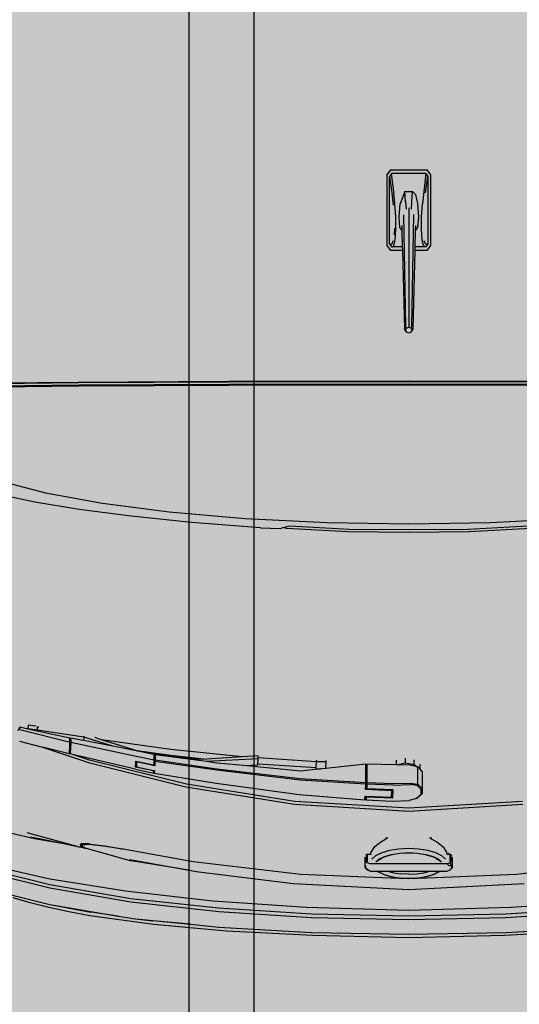
# Model space of a CAD drawing. Units: inches. Extents: x 1884 to 2398, y 474 to 1488.
# Tile 20 of 39: x 2308 to 2330, y 577 to 620. Entities that reach past the tile are written whole.
import ezdxf

# ---------------------------------------------------------------- set-up
doc = ezdxf.new("R2010")
doc.units = ezdxf.units.IN
doc.header["$MEASUREMENT"] = 0
doc.layers.get('0').update_dxf_attribs({"color": 250})
doc.layers.add('A-ANNO-DIMS', color=2, linetype='Continuous', lineweight=18)
doc.layers.add('C-VEHI', color=8, linetype='Continuous', lineweight=18)
doc.layers.add('Edges', color=250, linetype='Continuous')
doc.layers.add('L-PVMT-PATT', color=9, linetype='Continuous', lineweight=13, true_color=0xc7c8ca)
doc.styles.get("Standard").update_dxf_attribs({"font": 'arial.ttf'})
doc.dimstyles.get("Standard").update_dxf_attribs({"dimtxt": 7, "dimasz": 0.18, "dimexe": 0.18, "dimexo": 0.0625, "dimgap": 0.09, "dimtad": 0, "dimtih": 1, "dimtoh": 1, "dimzin": 0, "dimdsep": 46, "dimlunit": 3, "dimtxsty": 'Standard', "dimcen": 0.09, "dimadec": 0, "dimazin": 0, "dimtfac": 1, "dimtofl": 0, "dimtmove": 0, "dimatfit": 3, "dimfxl": 1, "dimtolj": 1, "dimtzin": 0, "dimarcsym": 0})

# ---------------------------------------------------------------- blocks, each defined once
blk = doc.blocks.new('Nissan Qashqai pl')
at = {"layer": 'Edges'}
for p, q in [((11.5963, 12.0406), (11.5823, 12.1589)), ((11.626, 12.1375), (11.6329, 12.0344)), ((11.6399, 12.029), (11.6333, 12.131)), ((11.6377, 12.1308), (11.6444, 12.0289)), ((11.6604, 12.0287), (11.6543, 12.1306)), ((11.0547, 11.9221), (11.0551, 12.1203)), ((11.0554, 11.9221), (11.0557, 12.1202)), ((11.0586, 12.1198), (11.0583, 11.9221)), ((11.0597, 12.1196), (11.0594, 11.9221)), ((11.6589, 12.1222), (11.6635, 12.0274)), ((11.2101, 12.012), (11.2057, 12.1019)), ((11.2168, 12.056), (11.2204, 11.989)), ((11.2174, 11.9874), (11.2139, 12.0528)), ((11.5166, 12.0471), (11.5239, 11.9221)), ((11.527, 11.9221), (11.5196, 12.0475)), ((11.6133, 11.9221), (11.6067, 12.0489)), ((11.6005, 11.9335), (11.5963, 12.0406)), ((11.6329, 12.0344), (11.6363, 11.9221)), ((11.6421, 11.9221), (11.6399, 12.029)), ((11.6444, 12.0289), (11.6465, 11.9221)), ((11.6623, 11.9221), (11.6604, 12.0287)), ((11.6635, 12.0274), (11.6663, 11.9221)), ((11.2116, 11.9221), (11.2101, 12.012)), ((11.218, 11.9221), (11.2174, 11.9874)), ((11.2204, 11.989), (11.2211, 11.9221)), ((11.5748, 11.9684), (11.5746, 11.9677)), ((11.5762, 11.9694), (11.5748, 11.9684)), ((11.5748, 11.9684), (11.5826, 11.9684)), ((11.5885, 11.9701), (11.5776, 11.9701)), ((11.5826, 11.9684), (11.5838, 11.9678)), ((11.5867, 11.9695), (11.5838, 11.9678)), ((11.5868, 11.966), (11.5867, 11.9695)), ((11.5896, 11.9695), (11.5867, 11.9695)), ((11.5885, 11.9701), (11.5896, 11.9695)), ((11.5915, 11.9678), (11.5896, 11.9695)), ((11.5915, 11.9678), (11.5904, 11.9684)), ((11.5608, 11.9528), (11.5659, 11.9594)), ((11.5659, 11.9594), (11.572, 11.9635)), ((11.572, 11.9635), (11.5746, 11.964)), ((11.5726, 11.9653), (11.5726, 11.9656)), ((11.5761, 11.9585), (11.5729, 11.9518)), ((11.5731, 11.9653), (11.5731, 11.9657)), ((11.5824, 11.9677), (11.5746, 11.9677)), ((11.5746, 11.9677), (11.5746, 11.964)), ((11.5746, 11.964), (11.5746, 11.9638)), ((11.5799, 11.9626), (11.5761, 11.9585)), ((11.5799, 11.9549), (11.5829, 11.9582)), ((11.5829, 11.9574), (11.58, 11.9542)), ((11.5838, 11.9678), (11.5851, 11.9645)), ((11.5868, 11.966), (11.5851, 11.9645)), ((11.5851, 11.9645), (11.5851, 11.8796)), ((11.5929, 11.9645), (11.5915, 11.9678)), ((11.5929, 11.9569), (11.5929, 11.9645)), ((11.5565, 11.9451), (11.5564, 11.9475)), ((11.5565, 11.9451), (11.5582, 11.9481)), ((11.5582, 11.9481), (11.5608, 11.9528)), ((11.5729, 11.9518), (11.5703, 11.9431)), ((11.5747, 11.941), (11.5769, 11.9489)), ((11.5771, 11.9483), (11.5749, 11.9407)), ((11.5769, 11.9489), (11.5799, 11.9549)), ((11.5788, 11.9517), (11.5771, 11.9483)), ((11.58, 11.9542), (11.5788, 11.9517)), ((11.5788, 11.9517), (11.58, 11.953)), ((11.5929, 11.9569), (11.5941, 11.9549)), ((11.5929, 11.9566), (11.5929, 11.9569)), ((11.5932, 11.9559), (11.5929, 11.9566)), ((11.5929, 11.9563), (11.5929, 11.9566)), ((11.5929, 11.9563), (11.5932, 11.9559)), ((11.5929, 11.9555), (11.5929, 11.9563)), ((11.594, 11.9542), (11.5929, 11.9555)), ((11.5929, 11.9453), (11.5929, 11.9555)), ((11.5932, 11.9559), (11.5941, 11.9549)), ((11.5969, 11.9483), (11.594, 11.9542)), ((11.5941, 11.9549), (11.5971, 11.9489)), ((11.5991, 11.9407), (11.5969, 11.9483)), ((11.5971, 11.9489), (11.5993, 11.941)), ((10.8228, 11.9421), (10.8224, 11.9421)), ((10.8228, 11.9421), (10.8283, 11.9461)), ((10.8228, 11.9021), (10.8228, 11.9421)), ((10.827, 11.9408), (10.8301, 11.9431)), ((10.827, 11.9408), (10.827, 11.9033)), ((10.827, 11.9408), (10.8467, 11.9386)), ((10.8279, 11.9461), (10.8283, 11.9461)), ((10.8283, 11.9461), (10.906, 11.9461)), ((10.8483, 11.9406), (10.8301, 11.9431)), ((10.8301, 11.9431), (10.9043, 11.9431)), ((10.8467, 11.9386), (10.8603, 11.9373)), ((10.8746, 11.9363), (10.8603, 11.9373)), ((10.8861, 11.9361), (10.8746, 11.9363)), ((10.8959, 11.9365), (10.8861, 11.9361)), ((10.9021, 11.9372), (10.8959, 11.9365)), ((10.9035, 11.9403), (10.9008, 11.9391)), ((10.9057, 11.9384), (10.9021, 11.9372)), ((10.905, 11.9414), (10.9035, 11.9403)), ((10.9043, 11.9431), (10.9074, 11.9408)), ((10.9043, 11.9431), (10.905, 11.9414)), ((10.9074, 11.9393), (10.9057, 11.9384)), ((10.906, 11.9461), (10.9116, 11.9421)), ((10.9074, 11.9408), (10.9074, 11.9393)), ((10.9074, 11.9393), (10.9074, 11.9291)), ((10.9116, 11.9421), (10.9116, 11.929)), ((11.4835, 11.937), (11.4811, 11.9346)), ((11.4835, 11.937), (11.5022, 11.937)), ((11.4974, 11.9321), (11.5022, 11.937)), ((11.5035, 11.9359), (11.4991, 11.9313)), ((11.5022, 11.937), (11.5081, 11.9367)), ((11.5089, 11.9356), (11.5035, 11.9359)), ((11.5081, 11.9367), (11.5129, 11.9312)), ((11.5089, 11.9356), (11.5132, 11.9305)), ((11.5703, 11.9431), (11.5688, 11.933)), ((11.5732, 11.9319), (11.5747, 11.941)), ((11.5749, 11.9407), (11.5735, 11.9317)), ((11.5929, 11.8989), (11.5929, 11.9453)), ((11.5948, 11.9386), (11.5929, 11.9453)), ((11.596, 11.9306), (11.5948, 11.9386)), ((11.6005, 11.9317), (11.5991, 11.9407)), ((11.5993, 11.941), (11.6005, 11.9335)), ((10.8467, 11.9263), (10.8501, 11.9295)), ((10.8467, 11.9178), (10.8467, 11.9263)), ((10.8579, 11.9255), (10.8467, 11.9263)), ((10.8501, 11.9295), (10.8603, 11.9316)), ((10.8662, 11.925), (10.8579, 11.9255)), ((10.8603, 11.9316), (10.8746, 11.9327)), ((10.9946, 11.9254), (10.872, 11.9276)), ((10.8746, 11.9327), (10.8861, 11.9319)), ((10.889, 11.9296), (10.884, 11.9298)), ((10.8861, 11.9319), (10.889, 11.9296)), ((10.9074, 11.9291), (10.889, 11.9296)), ((10.9116, 11.929), (10.9074, 11.9291)), ((10.9973, 11.9268), (10.9116, 11.929)), ((10.9969, 11.9247), (10.9946, 11.9254)), ((10.9969, 11.9247), (10.996, 11.9221)), ((10.999, 11.9258), (10.9969, 11.9247)), ((10.9973, 11.9268), (11.0001, 11.9254)), ((10.999, 11.9258), (10.9973, 11.9268)), ((11.0012, 11.9247), (10.999, 11.9258)), ((11.0012, 11.9247), (11.0001, 11.9254)), ((11.002, 11.9221), (11.0012, 11.9247)), ((11.4758, 11.928), (11.4706, 11.928)), ((11.474, 11.918), (11.4758, 11.928)), ((11.4811, 11.9346), (11.4755, 11.9346)), ((11.4758, 11.928), (11.4784, 11.9312)), ((11.4784, 11.9312), (11.4766, 11.9237)), ((11.4786, 11.9321), (11.4784, 11.9312)), ((11.4811, 11.9346), (11.4786, 11.9321)), ((11.4974, 11.9321), (11.4786, 11.9321)), ((11.4962, 11.9237), (11.4974, 11.9321)), ((11.4991, 11.9313), (11.498, 11.9236)), ((11.5132, 11.9305), (11.5129, 11.9312)), ((11.5132, 11.9305), (11.5154, 11.9227)), ((11.5688, 11.933), (11.5682, 11.9221)), ((11.5728, 11.9221), (11.5732, 11.9319)), ((11.5735, 11.9317), (11.573, 11.9221)), ((11.5964, 11.9221), (11.596, 11.9306)), ((11.6005, 11.9335), (11.6008, 11.9319)), ((11.601, 11.9221), (11.6005, 11.9317)), ((11.6008, 11.9319), (11.6012, 11.9221)), ((10.8579, 11.9187), (10.8467, 11.9178)), ((10.8467, 11.9178), (10.8603, 11.9126)), ((10.8579, 11.9187), (10.8662, 11.9191)), ((10.8647, 11.9221), (10.996, 11.9221)), ((10.8723, 11.9165), (10.9946, 11.9187)), ((10.884, 11.9144), (10.889, 11.9145)), ((10.889, 11.9145), (10.8861, 11.9122)), ((10.889, 11.9145), (10.9074, 11.915)), ((10.9074, 11.915), (10.9116, 11.9151)), ((10.9074, 11.915), (10.9074, 11.9049)), ((10.9116, 11.9151), (10.9973, 11.9173)), ((10.9116, 11.9151), (10.9116, 11.9021)), ((10.9946, 11.9187), (10.9969, 11.9195)), ((10.996, 11.9221), (10.9969, 11.9195)), ((10.9969, 11.9195), (10.999, 11.9184)), ((11.0001, 11.9187), (10.9973, 11.9173)), ((10.9973, 11.9173), (10.999, 11.9184)), ((10.999, 11.9184), (10.9996, 11.9187)), ((10.9996, 11.9187), (11.0012, 11.9195)), ((11.0001, 11.9187), (10.9996, 11.9187)), ((11.0012, 11.9195), (11.0001, 11.9187)), ((11.0012, 11.9195), (11.002, 11.9221)), ((11.0551, 11.7239), (11.0547, 11.9221)), ((11.0557, 11.724), (11.0554, 11.9221)), ((11.0583, 11.9221), (11.0586, 11.7244)), ((11.0594, 11.9221), (11.0597, 11.7245)), ((11.2101, 11.8322), (11.2116, 11.9221)), ((11.2174, 11.8567), (11.218, 11.9221)), ((11.2211, 11.9221), (11.2204, 11.8551)), ((11.469, 11.918), (11.474, 11.918)), ((11.4762, 11.9091), (11.474, 11.918)), ((11.4766, 11.9237), (11.4762, 11.9091)), ((11.4969, 11.9049), (11.4962, 11.9237)), ((11.4986, 11.9049), (11.498, 11.9236)), ((11.5161, 11.9039), (11.5154, 11.9227)), ((11.5239, 11.9221), (11.5166, 11.7971)), ((11.5196, 11.7967), (11.527, 11.9221)), ((11.5682, 11.9221), (11.5688, 11.9112)), ((11.5732, 11.9123), (11.5728, 11.9221)), ((11.573, 11.9221), (11.5735, 11.9125)), ((11.5964, 11.9221), (11.596, 11.9135)), ((11.6005, 11.9125), (11.601, 11.9221)), ((11.6012, 11.9221), (11.6008, 11.9123)), ((11.6067, 11.7952), (11.6133, 11.9221)), ((11.6363, 11.9221), (11.6329, 11.8098)), ((11.6399, 11.8152), (11.6421, 11.9221)), ((11.6465, 11.9221), (11.6444, 11.8153)), ((11.6604, 11.8154), (11.6623, 11.9221)), ((11.6663, 11.9221), (11.6635, 11.8168)), ((10.8467, 11.9056), (10.827, 11.9033)), ((10.827, 11.9033), (10.8301, 11.9011)), ((10.8301, 11.9011), (10.8483, 11.9036)), ((10.8603, 11.9068), (10.8467, 11.9056)), ((10.8483, 11.9036), (10.8619, 11.905)), ((10.8746, 11.9115), (10.8603, 11.9126)), ((10.8746, 11.9078), (10.8603, 11.9068)), ((10.8861, 11.9122), (10.8746, 11.9115)), ((10.8861, 11.908), (10.8746, 11.9078)), ((10.8959, 11.9077), (10.8861, 11.908)), ((10.8871, 11.9063), (10.8944, 11.906)), ((10.9021, 11.9069), (10.8959, 11.9077)), ((10.9008, 11.905), (10.9035, 11.9039)), ((10.9057, 11.9058), (10.9021, 11.9069)), ((10.9035, 11.9039), (10.905, 11.9028)), ((10.9043, 11.9011), (10.9074, 11.9033)), ((10.9074, 11.9049), (10.9057, 11.9058)), ((10.9074, 11.9033), (10.9074, 11.9049)), ((10.9074, 11.9033), (10.9074, 11.9048)), ((11.471, 11.9083), (11.4762, 11.9083)), ((11.4762, 11.9083), (11.4754, 11.8761)), ((11.4762, 11.9091), (11.4762, 11.9083)), ((11.4957, 11.8762), (11.4969, 11.9049)), ((11.4986, 11.9049), (11.4974, 11.8761)), ((11.5022, 11.8759), (11.5035, 11.9047)), ((11.5046, 11.9034), (11.5034, 11.8751)), ((11.5035, 11.9047), (11.513, 11.9041)), ((11.5118, 11.903), (11.5046, 11.9034)), ((11.513, 11.9041), (11.5118, 11.8754)), ((11.5148, 11.8751), (11.5161, 11.9039)), ((11.5688, 11.9112), (11.5703, 11.9011)), ((11.5747, 11.9032), (11.5732, 11.9123)), ((11.5735, 11.9125), (11.5749, 11.9035)), ((11.5769, 11.8953), (11.5747, 11.9032)), ((11.5749, 11.9035), (11.5771, 11.8958)), ((11.5929, 11.8989), (11.5948, 11.9056)), ((11.5948, 11.9056), (11.596, 11.9135)), ((11.5963, 11.8036), (11.6005, 11.9107)), ((11.5969, 11.8958), (11.5991, 11.9035)), ((11.5993, 11.9032), (11.5971, 11.8953)), ((11.5991, 11.9035), (11.6005, 11.9125)), ((11.6005, 11.9107), (11.5993, 11.9032)), ((11.6008, 11.9123), (11.6005, 11.9107)), ((10.8224, 11.9021), (10.8228, 11.9021)), ((10.8228, 11.9021), (10.8283, 11.8981)), ((10.8283, 11.8981), (10.8279, 11.8981)), ((10.8283, 11.8981), (10.906, 11.8981)), ((10.9043, 11.9011), (10.8301, 11.9011)), ((10.905, 11.9028), (10.9043, 11.9011)), ((10.906, 11.8981), (10.9116, 11.9021)), ((11.5106, 11.8751), (11.5118, 11.903)), ((11.5564, 11.8967), (11.5565, 11.8991)), ((11.5582, 11.896), (11.5565, 11.8991)), ((11.5608, 11.8913), (11.5582, 11.896)), ((11.5703, 11.9011), (11.5729, 11.8924)), ((11.5729, 11.8924), (11.5761, 11.8857)), ((11.5799, 11.8893), (11.5769, 11.8953)), ((11.5771, 11.8958), (11.5788, 11.8925)), ((11.58, 11.8912), (11.5788, 11.8925)), ((11.5788, 11.8925), (11.58, 11.8899)), ((11.5929, 11.8887), (11.5929, 11.8989)), ((11.594, 11.8899), (11.5969, 11.8958)), ((11.5971, 11.8953), (11.5941, 11.8893)), ((11.5659, 11.8848), (11.5608, 11.8913)), ((11.572, 11.8807), (11.5659, 11.8848)), ((11.5761, 11.8857), (11.5799, 11.8815)), ((11.5829, 11.886), (11.5799, 11.8893)), ((11.58, 11.8899), (11.5829, 11.8867)), ((11.5929, 11.8887), (11.594, 11.8899)), ((11.5929, 11.8872), (11.5941, 11.8893)), ((11.5929, 11.8879), (11.5929, 11.8887)), ((11.5929, 11.8876), (11.5932, 11.8883)), ((11.5932, 11.8883), (11.5929, 11.8879)), ((11.5929, 11.8876), (11.5929, 11.8879)), ((11.5929, 11.8872), (11.5929, 11.8876)), ((11.5929, 11.8796), (11.5929, 11.8872)), ((11.5941, 11.8893), (11.5932, 11.8883)), ((11.4754, 11.8761), (11.4945, 11.8762)), ((11.4956, 11.875), (11.4754, 11.8749)), ((11.4754, 11.8749), (11.4801, 11.831)), ((11.4913, 11.8028), (11.4956, 11.875)), ((11.4973, 11.8749), (11.493, 11.8027)), ((11.4945, 11.875), (11.4945, 11.8762)), ((11.4945, 11.8762), (11.4957, 11.8762)), ((11.5034, 11.8751), (11.4945, 11.875)), ((11.4973, 11.8749), (11.4956, 11.875)), ((11.4957, 11.8762), (11.4974, 11.8761)), ((11.5034, 11.8746), (11.4973, 11.8749)), ((11.4974, 11.8761), (11.5022, 11.8759)), ((11.5034, 11.8751), (11.5034, 11.8746)), ((11.5088, 11.8018), (11.5148, 11.8739)), ((11.5105, 11.8742), (11.5106, 11.8751)), ((11.5148, 11.8739), (11.5105, 11.8742)), ((11.5147, 11.8751), (11.5106, 11.8751)), ((11.5118, 11.8754), (11.5147, 11.8752)), ((11.5147, 11.8752), (11.5147, 11.8751)), ((11.5147, 11.8752), (11.5148, 11.8751)), ((11.5148, 11.8751), (11.5147, 11.8751)), ((11.5726, 11.8806), (11.572, 11.8807)), ((11.5726, 11.8806), (11.5726, 11.8808)), ((11.5731, 11.8805), (11.5726, 11.8806)), ((11.5731, 11.8805), (11.5731, 11.8808)), ((11.5746, 11.8802), (11.5731, 11.8805)), ((11.5746, 11.881), (11.5746, 11.8802)), ((11.5746, 11.8802), (11.5746, 11.8765)), ((11.5746, 11.8765), (11.5824, 11.8765)), ((11.5746, 11.8765), (11.5748, 11.8757)), ((11.5826, 11.8757), (11.5748, 11.8757)), ((11.5748, 11.8757), (11.5762, 11.8748)), ((11.5885, 11.8741), (11.5776, 11.8741)), ((11.5838, 11.8763), (11.5826, 11.8757)), ((11.5851, 11.8796), (11.5838, 11.8763)), ((11.5867, 11.8747), (11.5896, 11.8747)), ((11.5896, 11.8747), (11.5885, 11.8741)), ((11.5896, 11.8747), (11.5915, 11.8763)), ((11.5904, 11.8758), (11.5896, 11.8747)), ((11.5922, 11.8781), (11.5904, 11.8758)), ((11.5904, 11.8758), (11.5915, 11.8763)), ((11.5915, 11.8763), (11.5922, 11.8781)), ((11.5929, 11.8796), (11.5922, 11.8781)), ((11.2139, 11.7914), (11.2174, 11.8567)), ((11.2204, 11.8551), (11.2168, 11.7882)), ((11.2057, 11.7423), (11.2101, 11.8322)), ((11.473, 11.8314), (11.4716, 11.8314)), ((11.4801, 11.831), (11.473, 11.8314)), ((11.473, 11.8314), (11.473, 11.8209)), ((11.4801, 11.831), (11.4806, 11.8258)), ((11.4728, 11.8209), (11.4687, 11.7567)), ((11.4711, 11.8209), (11.4719, 11.8209)), ((11.4728, 11.8209), (11.4719, 11.8209)), ((11.473, 11.8209), (11.4728, 11.8209)), ((11.4792, 11.8205), (11.473, 11.8209)), ((11.4751, 11.7564), (11.4792, 11.8205)), ((11.4806, 11.8204), (11.4792, 11.8205)), ((11.4792, 11.8205), (11.4792, 11.8205)), ((11.4806, 11.8204), (11.4806, 11.8258)), ((11.4806, 11.8258), (11.4831, 11.803)), ((11.6635, 11.8168), (11.6589, 11.7219)), ((11.6329, 11.8098), (11.626, 11.7067)), ((11.6333, 11.7132), (11.6399, 11.8152)), ((11.6444, 11.8153), (11.6377, 11.7134)), ((11.6543, 11.7136), (11.6604, 11.8154)), ((11.4831, 11.803), (11.4771, 11.7404)), ((11.4805, 11.7113), (11.4913, 11.8028)), ((11.493, 11.8027), (11.4821, 11.7112)), ((11.4964, 11.7104), (11.5088, 11.8018)), ((11.5166, 11.7971), (11.4976, 11.678)), ((11.5005, 11.6772), (11.5196, 11.7967)), ((11.5823, 11.6852), (11.5963, 11.8036)), ((11.5932, 11.6885), (11.6067, 11.7952)), ((11.2158, 11.7842), (11.2139, 11.7914)), ((11.2168, 11.7882), (11.2158, 11.784)), ((11.2168, 11.7882), (11.2158, 11.7842)), ((11.2158, 11.784), (11.2158, 11.7842)), ((11.2166, 11.7812), (11.2158, 11.784)), ((11.2159, 11.7591), (11.2166, 11.7812)), ((11.2159, 11.7591), (11.21, 11.6835)), ((11.4687, 11.7567), (11.4665, 11.7568)), ((11.4665, 11.7568), (11.4676, 11.7389)), ((11.4698, 11.7567), (11.4687, 11.7567)), ((11.4698, 11.7567), (11.4727, 11.6999)), ((11.4751, 11.7564), (11.4698, 11.7567)), ((11.4761, 11.7564), (11.4751, 11.7564)), ((11.4771, 11.7404), (11.4761, 11.7564)), ((11.1984, 11.6587), (11.2057, 11.7423)), ((11.4676, 11.7389), (11.4594, 11.6607)), ((11.4676, 11.7389), (11.4699, 11.7001)), ((11.4771, 11.7404), (11.4743, 11.7114)), ((11.056, 11.559), (11.0551, 11.7239)), ((11.0566, 11.5593), (11.0557, 11.724)), ((11.0586, 11.7244), (11.0595, 11.5599)), ((11.0597, 11.7245), (11.0606, 11.5601)), ((11.6589, 11.7219), (11.6514, 11.6415)), ((11.4709, 11.6433), (11.4805, 11.7113)), ((11.4821, 11.7112), (11.4726, 11.6432)), ((11.4743, 11.7114), (11.4727, 11.6999)), ((11.4854, 11.6425), (11.4964, 11.7104)), ((11.6229, 11.6168), (11.6333, 11.7132)), ((11.6377, 11.7134), (11.6272, 11.6169)), ((11.6511, 11.6823), (11.6543, 11.7136)), ((11.4727, 11.6999), (11.4651, 11.6434)), ((11.4658, 11.6603), (11.4699, 11.7001)), ((11.4699, 11.7001), (11.4705, 11.6909)), ((11.626, 11.7067), (11.615, 11.6108)), ((11.4705, 11.6909), (11.4642, 11.6385)), ((11.5922, 11.6828), (11.5932, 11.6885)), ((11.21, 11.6835), (11.2033, 11.6172)), ((11.4976, 11.678), (11.4712, 11.5713)), ((11.4738, 11.5702), (11.5005, 11.6772)), ((11.5685, 11.6083), (11.5823, 11.6852)), ((11.5802, 11.6156), (11.5922, 11.6828)), ((11.5922, 11.6828), (11.5818, 11.6172)), ((11.6448, 11.6184), (11.6511, 11.6823)), ((11.6511, 11.6823), (11.6475, 11.6409)), ((11.1891, 11.5856), (11.1984, 11.6587)), ((11.4594, 11.6607), (11.4487, 11.5846)), ((11.4602, 11.6212), (11.4658, 11.6603)), ((11.4642, 11.6385), (11.4611, 11.6241)), ((11.4651, 11.6426), (11.4642, 11.6385)), ((11.4651, 11.6434), (11.468, 11.6433)), ((11.4679, 11.6425), (11.4651, 11.6426)), ((11.4669, 11.6225), (11.4709, 11.6424)), ((11.468, 11.6433), (11.4679, 11.6425)), ((11.4709, 11.6424), (11.4679, 11.6425)), ((11.468, 11.6433), (11.4709, 11.6433)), ((11.4709, 11.6433), (11.4726, 11.6432)), ((11.4725, 11.6423), (11.4709, 11.6424)), ((11.4721, 11.6222), (11.4763, 11.6421)), ((11.4744, 11.6422), (11.4725, 11.6423)), ((11.4726, 11.6432), (11.4745, 11.6431)), ((11.4773, 11.643), (11.4731, 11.6231)), ((11.4744, 11.6422), (11.4745, 11.6431)), ((11.4763, 11.6421), (11.4744, 11.6422)), ((11.4745, 11.6431), (11.4773, 11.643)), ((11.4783, 11.6228), (11.4823, 11.6417)), ((11.483, 11.6417), (11.4788, 11.6219)), ((11.481, 11.6217), (11.4853, 11.6416)), ((11.4823, 11.6417), (11.4824, 11.6425)), ((11.4823, 11.6417), (11.483, 11.6417)), ((11.4824, 11.6425), (11.4825, 11.6427)), ((11.4853, 11.6425), (11.4824, 11.6425)), ((11.4825, 11.6427), (11.4853, 11.6425)), ((11.4853, 11.6416), (11.483, 11.6418)), ((11.483, 11.6418), (11.483, 11.6417)), ((11.4854, 11.6425), (11.4853, 11.6425)), ((11.6514, 11.6415), (11.6422, 11.5716)), ((11.6448, 11.6184), (11.6475, 11.6409)), ((11.4513, 11.5507), (11.4669, 11.6225)), ((11.4608, 11.6226), (11.4558, 11.5969)), ((11.4611, 11.6241), (11.4602, 11.6212)), ((11.4611, 11.6241), (11.4608, 11.6226)), ((11.4749, 11.6221), (11.4721, 11.6222)), ((11.4731, 11.6231), (11.4751, 11.6229)), ((11.4749, 11.6221), (11.4751, 11.6229)), ((11.4788, 11.6219), (11.4749, 11.6221)), ((11.4751, 11.6229), (11.4783, 11.6228)), ((11.2033, 11.6172), (11.1958, 11.5598)), ((11.4602, 11.6212), (11.4487, 11.5846)), ((11.481, 11.6217), (11.4649, 11.5526)), ((11.5678, 11.5675), (11.5818, 11.6172)), ((11.6076, 11.5276), (11.6229, 11.6168)), ((11.6272, 11.6169), (11.6118, 11.5276)), ((11.6423, 11.603), (11.6446, 11.6171)), ((11.6446, 11.6171), (11.6448, 11.6184)), ((11.565, 11.5864), (11.5685, 11.6083)), ((11.5691, 11.6089), (11.5656, 11.5882)), ((11.615, 11.6108), (11.6016, 11.5276)), ((11.6301, 11.53), (11.6423, 11.603)), ((11.6423, 11.603), (11.6381, 11.5726)), ((11.4558, 11.5969), (11.4458, 11.5652)), ((11.4558, 11.5969), (11.4496, 11.5649)), ((11.1776, 11.5231), (11.1891, 11.5856)), ((11.4472, 11.5801), (11.4464, 11.5774)), ((11.4487, 11.5846), (11.4472, 11.5801)), ((11.5636, 11.5736), (11.565, 11.5864)), ((11.5656, 11.5882), (11.5641, 11.5754)), ((11.4568, 11.5197), (11.4738, 11.5702)), ((11.4712, 11.5713), (11.4649, 11.5526)), ((11.5627, 11.5696), (11.5626, 11.5697)), ((11.5626, 11.567), (11.5627, 11.5696)), ((11.5627, 11.5696), (11.5628, 11.5721)), ((11.5634, 11.5684), (11.5627, 11.5696)), ((11.5632, 11.5659), (11.5634, 11.5684)), ((11.5634, 11.5684), (11.5636, 11.5736)), ((11.5637, 11.5679), (11.5634, 11.5684)), ((11.5641, 11.5754), (11.5638, 11.5679)), ((11.5638, 11.5679), (11.5639, 11.5632)), ((11.6301, 11.53), (11.6381, 11.5726)), ((11.6422, 11.5716), (11.6375, 11.5486)), ((11.0572, 11.4499), (11.056, 11.559)), ((11.0579, 11.4504), (11.0566, 11.5593)), ((11.0595, 11.5599), (11.0607, 11.4508)), ((11.0606, 11.5601), (11.0618, 11.4509)), ((11.1958, 11.5598), (11.1877, 11.5111)), ((11.4458, 11.5652), (11.438, 11.514)), ((11.4448, 11.5652), (11.4458, 11.5652)), ((11.4458, 11.5652), (11.4496, 11.5649)), ((11.4458, 11.5652), (11.4458, 11.5652)), ((11.4496, 11.5649), (11.4468, 11.5505)), ((11.5505, 11.5023), (11.5665, 11.5614)), ((11.5627, 11.5624), (11.5626, 11.567)), ((11.5633, 11.5627), (11.5627, 11.5624)), ((11.5634, 11.5613), (11.5627, 11.5624)), ((11.5627, 11.5431), (11.5665, 11.5614)), ((11.5633, 11.5627), (11.5632, 11.5659)), ((11.5661, 11.5639), (11.5633, 11.5627)), ((11.5634, 11.5613), (11.5633, 11.5627)), ((11.5658, 11.5622), (11.5634, 11.5613)), ((11.5639, 11.5632), (11.5643, 11.5634)), ((11.5643, 11.5634), (11.566, 11.5641)), ((11.5649, 11.5659), (11.5647, 11.5662)), ((11.5661, 11.5639), (11.5658, 11.5622)), ((11.5662, 11.5624), (11.5658, 11.5622)), ((11.566, 11.5641), (11.5662, 11.5642)), ((11.5661, 11.5639), (11.566, 11.5641)), ((11.5662, 11.5642), (11.5661, 11.5639)), ((11.5661, 11.5639), (11.5662, 11.5642)), ((11.5661, 11.5639), (11.5665, 11.5641)), ((11.5661, 11.5639), (11.5661, 11.5639)), ((11.5662, 11.5642), (11.5665, 11.5643)), ((11.5667, 11.5642), (11.5662, 11.5624)), ((11.5662, 11.5642), (11.5662, 11.5642)), ((11.5662, 11.5624), (11.5665, 11.5641)), ((11.5666, 11.5625), (11.5662, 11.5624)), ((11.5665, 11.5643), (11.5667, 11.5644)), ((11.5665, 11.5641), (11.5665, 11.5643)), ((11.5665, 11.5641), (11.5667, 11.5642)), ((11.5668, 11.5626), (11.5665, 11.5614)), ((11.5666, 11.5625), (11.567, 11.5645)), ((11.5667, 11.5626), (11.5666, 11.5625)), ((11.5667, 11.5626), (11.5671, 11.5646)), ((11.5667, 11.5644), (11.5669, 11.5645)), ((11.5667, 11.5642), (11.5669, 11.5645)), ((11.5667, 11.5644), (11.5667, 11.5642)), ((11.5668, 11.5626), (11.5667, 11.5626)), ((11.5672, 11.5646), (11.5668, 11.5626)), ((11.5669, 11.5645), (11.567, 11.5645)), ((11.567, 11.5645), (11.5674, 11.5662)), ((11.567, 11.5645), (11.5671, 11.5646)), ((11.5671, 11.5646), (11.5676, 11.5671)), ((11.5671, 11.5646), (11.5672, 11.5646)), ((11.5672, 11.5646), (11.5676, 11.5671)), ((11.5675, 11.5665), (11.5674, 11.5662)), ((11.5676, 11.5671), (11.5678, 11.5675)), ((11.4375, 11.4946), (11.4512, 11.5499)), ((11.4468, 11.5496), (11.4391, 11.5139)), ((11.4468, 11.5505), (11.45, 11.5507)), ((11.4498, 11.5498), (11.4468, 11.5496)), ((11.4498, 11.5498), (11.45, 11.5507)), ((11.4512, 11.5499), (11.4498, 11.5498)), ((11.45, 11.5507), (11.4513, 11.5507)), ((11.4529, 11.5498), (11.4512, 11.5499)), ((11.4513, 11.5507), (11.4529, 11.5507)), ((11.4529, 11.5507), (11.4571, 11.5505)), ((11.4571, 11.5496), (11.4529, 11.5498)), ((11.4643, 11.5491), (11.4568, 11.5197)), ((11.4571, 11.5505), (11.4599, 11.5503)), ((11.462, 11.5493), (11.4571, 11.5496)), ((11.4598, 11.5498), (11.4599, 11.5503)), ((11.464, 11.55), (11.4598, 11.5498)), ((11.4599, 11.5503), (11.462, 11.5502)), ((11.462, 11.5502), (11.464, 11.55)), ((11.4638, 11.5492), (11.462, 11.5493)), ((11.464, 11.55), (11.4638, 11.5492)), ((11.4643, 11.5491), (11.4638, 11.5492)), ((11.464, 11.55), (11.464, 11.55)), ((11.4642, 11.55), (11.464, 11.55)), ((11.464, 11.55), (11.4642, 11.55)), ((11.4642, 11.55), (11.4642, 11.55)), ((11.4643, 11.55), (11.4642, 11.55)), ((11.4649, 11.5526), (11.4643, 11.55)), ((11.6375, 11.5486), (11.6328, 11.5267)), ((11.5553, 11.5068), (11.5627, 11.5431)), ((11.5571, 11.511), (11.5627, 11.5431)), ((11.6016, 11.5276), (11.5866, 11.4607)), ((11.5884, 11.4499), (11.6076, 11.5276)), ((11.6118, 11.5276), (11.5922, 11.4494)), ((11.6127, 11.4589), (11.6297, 11.5276)), ((11.6328, 11.5267), (11.6277, 11.5063)), ((11.6297, 11.5276), (11.6301, 11.53)), ((11.164, 11.4711), (11.1776, 11.5231)), ((11.4347, 11.5141), (11.434, 11.5141)), ((11.435, 11.5158), (11.4347, 11.5141)), ((11.438, 11.514), (11.4347, 11.5141)), ((11.4382, 11.514), (11.4368, 11.5036)), ((11.4391, 11.5139), (11.4369, 11.5036)), ((11.4382, 11.514), (11.438, 11.514)), ((11.4391, 11.5139), (11.4382, 11.514)), ((11.4503, 11.4945), (11.4568, 11.5197)), ((11.1877, 11.5111), (11.1791, 11.4696)), ((11.4337, 11.5124), (11.4325, 11.5038)), ((11.4325, 11.5038), (11.4368, 11.5036)), ((11.4325, 11.5038), (11.4369, 11.5035)), ((11.4369, 11.5035), (11.435, 11.4947)), ((11.4368, 11.5036), (11.4369, 11.5036)), ((11.4369, 11.5036), (11.4369, 11.5035)), ((11.5481, 11.471), (11.5571, 11.511)), ((11.6277, 11.5063), (11.6224, 11.4874)), ((11.435, 11.4947), (11.439, 11.4927)), ((11.4375, 11.4946), (11.435, 11.4947))]:
    blk.add_line(p, q, dxfattribs=at)
blk = doc.blocks.new('car')
blk.add_blockref('Nissan Qashqai pl', (-9.7433, -11.9151))
blk = doc.blocks.new('carr')
blk.add_blockref('car', (0.5124, -0.007))
blk = doc.blocks.new('*D23')
at = {"layer": 'A-ANNO-DIMS', "color": 0, "lineweight": -2, "transparency": 16777216}
for p, q in [((2272.304, 752.812), (2298.291, 752.812)), ((2298.111, 752.632), (2298.111, 670.29)), ((2298.111, 580.529), (2298.111, 662.871)), ((2272.304, 580.349), (2298.291, 580.349))]:
    blk.add_line(p, q, dxfattribs=at)
at = {"layer": 'A-ANNO-DIMS', "color": 0, "lineweight": 100, "transparency": 16777216}
for points in [[(2298.081, 752.632), (2298.141, 752.632), (2298.111, 752.812)], [(2298.081, 580.529), (2298.141, 580.529), (2298.111, 580.349)]]:
    blk.add_solid(points, dxfattribs=at)
at = {"layer": 'Defpoints', "color": 0, "lineweight": 100, "transparency": 16777216}
for p in [(2272.242, 752.812), (2272.242, 580.349), (2298.111, 580.349)]:
    blk.add_point(p, dxfattribs=at)
at = {"layer": 'A-ANNO-DIMS', "color": 0, "transparency": 16777216, "insert": (2298.111, 666.58), "char_height": 7, "attachment_point": 5}
blk.add_mtext('\\A1;CAR 14\'-4 1/2" TYP.', dxfattribs=at)
blk = doc.blocks.new('*D47')
at = {"layer": 'A-ANNO-DIMS', "color": 0, "lineweight": -2, "transparency": 16777216}
for p, q in [((2315.591, 959.704), (2315.591, 484.005)), ((2342.529, 959.704), (2342.529, 484.005)), ((2315.771, 484.185), (2319.606, 484.185)), ((2342.349, 484.185), (2338.513, 484.185))]:
    blk.add_line(p, q, dxfattribs=at)
at = {"layer": 'A-ANNO-DIMS', "color": 0, "lineweight": 100, "transparency": 16777216}
for points in [[(2315.771, 484.215), (2315.771, 484.155), (2315.591, 484.185)], [(2342.349, 484.215), (2342.349, 484.155), (2342.529, 484.185)]]:
    blk.add_solid(points, dxfattribs=at)
at = {"layer": 'Defpoints', "color": 0, "lineweight": 100, "transparency": 16777216}
for p in [(2315.591, 959.766), (2342.529, 959.766), (2342.529, 484.185)]:
    blk.add_point(p, dxfattribs=at)
at = {"layer": 'A-ANNO-DIMS', "color": 0, "transparency": 16777216, "insert": (2329.06, 484.185), "char_height": 7, "attachment_point": 5}
blk.add_mtext('\\A1;2\'-3"', dxfattribs=at)
blk = doc.blocks.new('*D49')
at = {"layer": 'A-ANNO-DIMS', "color": 0, "lineweight": -2, "transparency": 16777216}
for p, q in [((2318.409, 987.716), (2318.409, 484.005)), ((2340.409, 987.716), (2340.409, 484.005)), ((2318.589, 484.185), (2340.229, 484.185)), ((2340.409, 484.185), (2340.589, 484.185))]:
    blk.add_line(p, q, dxfattribs=at)
at = {"layer": 'A-ANNO-DIMS', "color": 0, "lineweight": 100, "transparency": 16777216}
for points in [[(2318.589, 484.215), (2318.589, 484.155), (2318.409, 484.185)], [(2340.229, 484.215), (2340.229, 484.155), (2340.409, 484.185)]]:
    blk.add_solid(points, dxfattribs=at)
at = {"layer": 'Defpoints', "color": 0, "lineweight": 100, "transparency": 16777216}
for p in [(2318.409, 987.778), (2340.409, 987.778), (2340.409, 484.185)]:
    blk.add_point(p, dxfattribs=at)
at = {"layer": 'A-ANNO-DIMS', "color": 0, "transparency": 16777216, "insert": (2352.373, 484.185), "char_height": 7, "attachment_point": 5}
blk.add_mtext('\\A1;1\'-10"', dxfattribs=at)

msp = doc.modelspace()

# ---------------------------------------------------------------- hatches: boundary and pattern name
at = {"layer": 'L-PVMT-PATT'}
h = msp.add_hatch(color=256, dxfattribs=at)
h.dxf.hatch_style = 1
h.paths.add_polyline_path([(2387.529, 769.966), (2351.529, 769.966), (2238.447, 769.966), (2238.447, 762.15), (2238.447, 754.445), (2126.529, 754.445), (2126.529, 676.183), (2134.868, 676.183), (2142.673, 676.183), (2142.673, 646.578), (2134.868, 646.578), (2126.529, 646.578), (2126.529, 640.17), (2387.529, 640.17)])
h.paths.add_polyline_path([(2387.529, 631.385), (2303.086, 631.385), (2303.086, 615.671), (2387.529, 615.671)])
h.paths.add_polyline_path([(2387.529, 640.17), (2126.529, 640.17), (2126.529, 631.385), (2387.529, 631.385)])
h.paths.add_polyline_path([(2393.529, 604.13), (2387.529, 604.13), (2387.529, 615.671), (2303.086, 615.671), (2303.086, 607.943), (2249.649, 607.943), (2126.529, 607.943), (2126.529, 533.885), (2393.529, 533.885)])
h.paths.add_polyline_path([(2257.825, 611.008), (2257.83, 611.337), (2257.915, 616.493), (2258.021, 621.805), (2258.146, 627.274), (2258.252, 631.385), (2126.529, 631.385), (2126.529, 611.008)])
h.paths.add_polyline_path([(2258.892, 611.285), (2258.888, 611.008), (2300.247, 611.008), (2300.247, 631.385), (2259.314, 631.385), (2259.206, 627.173), (2259.081, 621.72), (2258.976, 616.424)])

# ---------------------------------------------------------------- block references
at = {"layer": 'C-VEHI', "xscale": 39.37007874015748, "yscale": 39.37007874015748, "zscale": 39.37007874015748, "rotation": 270}
msp.add_blockref('carr', (2325.111, 676.232), dxfattribs=at)

# ---------------------------------------------------------------- dimensions: what is measured, and where the dimension line sits
at = {"layer": 'A-ANNO-DIMS'}
for base, p1, p2, picture, middle in [((2340.409, 484.185), (2318.409, 987.778), (2340.409, 987.778), '*D49', (2352.373, 484.185)), ((2342.529, 484.185), (2315.591, 959.766), (2342.529, 959.766), '*D47', (2329.06, 484.185))]:
    dim = msp.add_linear_dim(base=base, p1=p1, p2=p2, dimstyle='Standard', override={"dimdec": 1, "dimlfac": 1, "dimrnd": 0, "dimzin": 1, "dimdsep": 46, "dimlunit": 4, "dimfrac": 2}, dxfattribs=at)
    dim.commit()
    dim.dimension.update_dxf_attribs({"geometry": picture, "text_midpoint": middle})
dim = msp.add_linear_dim(base=(2298.111, 580.349), p1=(2272.242, 752.812), p2=(2272.242, 580.349), angle=270, text='CAR <> TYP.', dimstyle='Standard', override={"dimdec": 1, "dimlfac": 1, "dimrnd": 0, "dimzin": 1, "dimdsep": 46, "dimlunit": 4, "dimfrac": 2}, dxfattribs=at)
dim.commit()
dim.dimension.update_dxf_attribs({"geometry": '*D23', "text_midpoint": (2298.111, 666.58)})

doc.saveas('drawing.dxf')
